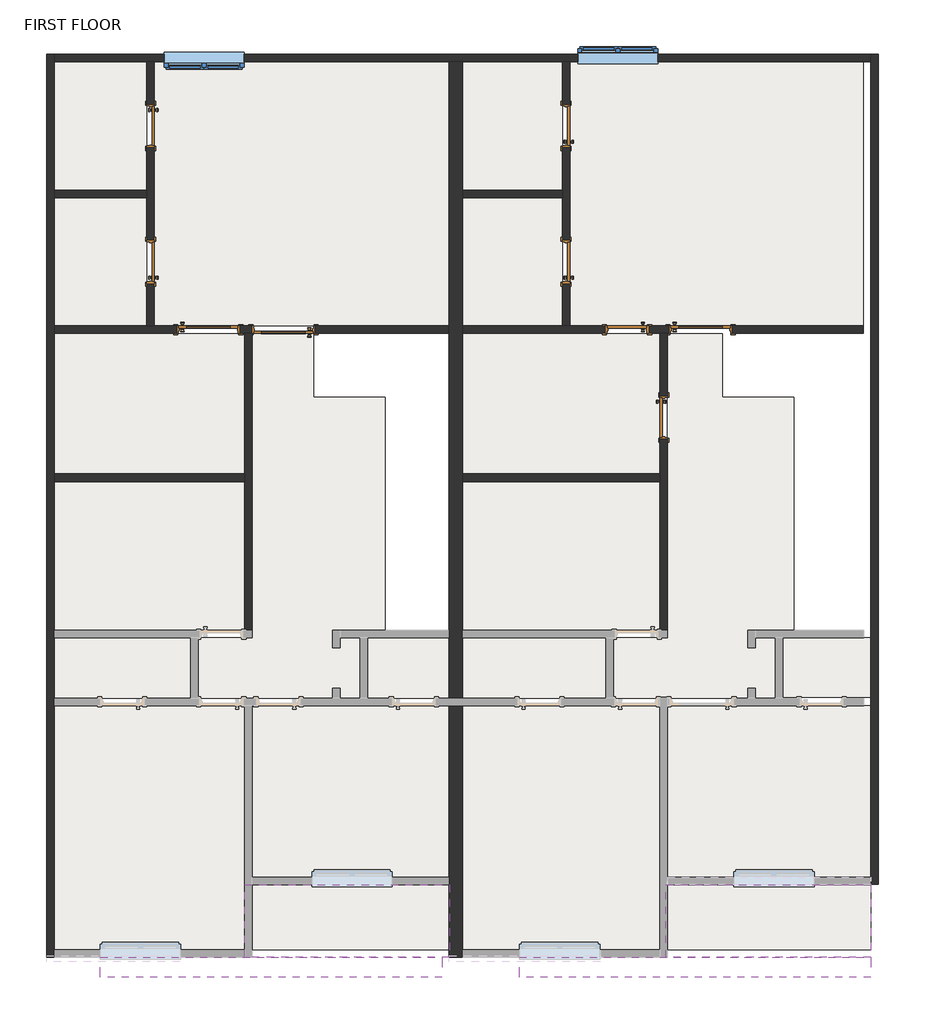
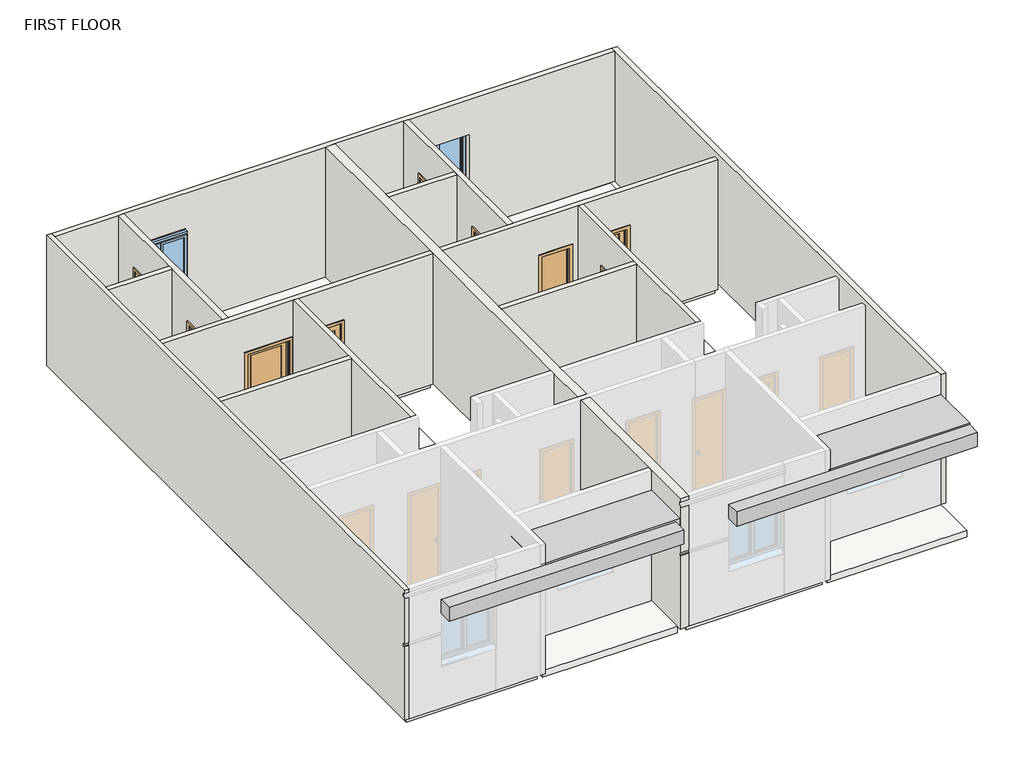
# One storey, part 2 of 2: 14 walls, 9 doors, 4 proxies, 2 slabs, 2 windows, 1 beam.
"""IFC4 building model written with IfcOpenShell, lengths in millimetres."""

from ifc_helpers import new_model, si_unit, frame, origin, place, context, project, spatial, polyline, outline, extrude, faceted_brep, transform, mapped, element, save
from components import w_shapes_w12x26_f1af6e5e, generic_models_1_generic_models_1_a2adb7c9, generic_models_2_generic_models_2_3446db89, generic_models_4_generic_models_1_d4ed459b, door_d4071c8b, door_c25f678d, door_03233f92, w2_0001_w2_3_7b164e2c

model = new_model("IFC4")

# Units and contexts
model_context = context("Model", 3, world=origin())
ifc_project = project(units=[si_unit("LENGTHUNIT", "METRE", prefix="MILLI")], contexts=[model_context])

# Site, building, storey
site = spatial("IfcSite", under=ifc_project)
building = spatial("IfcBuilding", under=site)
storey = spatial("IfcBuildingStorey", under=building, Name="FIRST FLOOR", Elevation=3352.8)

# Beam
placement = place(None, origin())
w_shapes_w12x26_shape = w_shapes_w12x26_f1af6e5e(model_context)
element("IfcBeam", 1, ObjectType="W Shapes : W12X26", at=placement, inside=storey, context=model_context, shape_type="MappedRepresentation", body=[
    mapped(w_shapes_w12x26_shape, transform((-13919.8007021, -597.2590801, 3197.86), x_axis=(0.0, 1.0, 0.0), y_axis=(-1.0, 0.0, 0.0), z_axis=(0.0, 0.0, 1.0))),
])

# Proxies
generic_models_1_generic_models_1_shape = generic_models_1_generic_models_1_a2adb7c9(model_context)
element("IfcBuildingElementProxy", 2, Name="Generic Models 1 : Generic Models 1", ObjectType="Generic Models 1 : Generic Models 1", at=placement, inside=storey, context=model_context, shape_type="MappedRepresentation", body=[
    mapped(generic_models_1_generic_models_1_shape, transform((0.0, 0.0, 0.0), x_axis=(1.0, 0.0, 0.0), y_axis=(0.0, 1.0, 0.0), z_axis=(0.0, 0.0, 1.0))),
])
generic_models_2_generic_models_2_shape = generic_models_2_generic_models_2_3446db89(model_context)
element("IfcBuildingElementProxy", 3, Name="Generic Models 2 : Generic Models 2", ObjectType="Generic Models 2 : Generic Models 2", at=placement, inside=storey, context=model_context, shape_type="MappedRepresentation", body=[
    mapped(generic_models_2_generic_models_2_shape, transform((0.0, 0.0, 0.0), x_axis=(1.0, 0.0, 0.0), y_axis=(0.0, 1.0, 0.0), z_axis=(0.0, 0.0, 1.0))),
])
element("IfcBuildingElementProxy", 4, Name="Generic Models 3 : Generic Models 2", ObjectType="Generic Models 3 : Generic Models 2", at=placement, inside=storey, context=model_context, shape_type="MappedRepresentation", body=[
    mapped(generic_models_2_generic_models_2_shape, transform((6400.8, 0.0, 0.0), x_axis=(1.0, 0.0, 0.0), y_axis=(0.0, 1.0, 0.0), z_axis=(0.0, 0.0, 1.0))),
])
generic_models_4_generic_models_1_shape = generic_models_4_generic_models_1_d4ed459b(model_context)
element("IfcBuildingElementProxy", 5, Name="Generic Models 4 : Generic Models 1", ObjectType="Generic Models 4 : Generic Models 1", at=placement, inside=storey, context=model_context, shape_type="MappedRepresentation", body=[
    mapped(generic_models_4_generic_models_1_shape, transform((6368.5786506, 0.0, 0.0), x_axis=(1.0, 0.0, 0.0), y_axis=(0.0, 1.0, 0.0), z_axis=(0.0, 0.0, 1.0))),
])

# Doors
door_shape = door_d4071c8b(model_context)
element("IfcDoor", 6, ObjectType="Door-Interior-Single-2_Panel-Wood : 36\" x 84\"", at=placement, inside=storey, context=model_context, shape_type="MappedRepresentation", body=[
    mapped(door_shape, transform((-14662.7507021, 4098.5659199, 3352.8), x_axis=(-1.0, 0.0, 0.0), y_axis=(0.0, -1.0, 0.0), z_axis=(0.0, 0.0, 1.0))),
])
element("IfcDoor", 7, ObjectType="Door-Interior-Single-2_Panel-Wood : 36\" x 84\"", at=placement, inside=storey, context=model_context, shape_type="MappedRepresentation", body=[
    mapped(door_shape, transform((-15805.7507021, 4104.9159199, 3352.8), x_axis=(1.0, 0.0, 0.0), y_axis=(0.0, 1.0, 0.0), z_axis=(0.0, 0.0, 1.0))),
])
element("IfcDoor", 8, ObjectType="Door-Interior-Single-2_Panel-Wood : 36\" x 84\"", at=placement, inside=storey, context=model_context, shape_type="MappedRepresentation", body=[
    mapped(door_shape, transform((-8325.4507021, 4104.9159199, 3352.8), x_axis=(1.0, 0.0, 0.0), y_axis=(0.0, 1.0, 0.0), z_axis=(0.0, 0.0, 1.0))),
])
door_2_shape = door_c25f678d(model_context)
element("IfcDoor", 9, ObjectType="Door-Interior-Single-Flush_Panel-Wood : 24\" x 84\"", at=placement, inside=storey, context=model_context, shape_type="MappedRepresentation", body=[
    mapped(door_2_shape, transform((-16678.8757021, 7197.3659199, 3352.8), x_axis=(0.0, -1.0, 0.0), y_axis=(1.0, 0.0, 0.0), z_axis=(0.0, 0.0, 1.0))),
])
door_3_shape = door_03233f92(model_context)
element("IfcDoor", 10, ObjectType="Door-Interior-Single-Flush_Panel-Wood : 24\" x 84\"", at=placement, inside=storey, context=model_context, shape_type="MappedRepresentation", body=[
    mapped(door_3_shape, transform((-16678.8757021, 5133.6159199, 3352.8), x_axis=(0.0, 1.0, 0.0), y_axis=(-1.0, 0.0, 0.0), z_axis=(0.0, 0.0, 1.0))),
])
element("IfcDoor", 11, ObjectType="Door-Interior-Single-Flush_Panel-Wood : 24\" x 84\"", at=placement, inside=storey, context=model_context, shape_type="MappedRepresentation", body=[
    mapped(door_3_shape, transform((-10366.9757021, 5133.6159199, 3352.8), x_axis=(0.0, 1.0, 0.0), y_axis=(-1.0, 0.0, 0.0), z_axis=(0.0, 0.0, 1.0))),
])
element("IfcDoor", 12, ObjectType="Door-Interior-Single-Flush_Panel-Wood : 24\" x 84\"", at=placement, inside=storey, context=model_context, shape_type="MappedRepresentation", body=[
    mapped(door_3_shape, transform((-10366.9757021, 7197.3659199, 3352.8), x_axis=(0.0, 1.0, 0.0), y_axis=(-1.0, 0.0, 0.0), z_axis=(0.0, 0.0, 1.0))),
])
element("IfcDoor", 13, ObjectType="Door-Interior-Single-Flush_Panel-Wood : 24\" x 84\"", at=placement, inside=storey, context=model_context, shape_type="MappedRepresentation", body=[
    mapped(door_3_shape, transform((-8887.4257021, 2768.2409199, 3352.8), x_axis=(0.0, -1.0, 0.0), y_axis=(1.0, 0.0, 0.0), z_axis=(0.0, 0.0, 1.0))),
])
element("IfcDoor", 14, ObjectType="Door-Interior-Single-Flush_Panel-Wood : 24\" x 84\"", at=placement, inside=storey, context=model_context, shape_type="MappedRepresentation", body=[
    mapped(door_3_shape, transform((-9443.0507021, 4104.9159199, 3352.8), x_axis=(-1.0, 0.0, 0.0), y_axis=(0.0, -1.0, 0.0), z_axis=(0.0, 0.0, 1.0))),
])

# Slabs
element("IfcSlab", 15, ObjectType="Generic - 12\" 2", at=placement, inside=storey, context=model_context, shape_type="SweptSolid", body=[
    extrude(outline(polyline([(-16739.2007021, 8172.0909199), (-16739.2007021, 6222.6409199), (-18148.9007021, 6222.6409199), (-18148.9007021, 8172.0909199), (-16739.2007021, 8172.0909199)])), frame((0.0, 0.0, 3200.4), z_axis=(0.0, 0.0, 1.0), x_axis=(1.0, 0.0, 0.0)), (0.0, 0.0, 1.0), 152.4),
    extrude(outline(polyline([(-16739.2007021, 6108.3409199), (-16739.2007021, 4158.8909199), (-18148.9007021, 4158.8909199), (-18148.9007021, 6108.3409199), (-16739.2007021, 6108.3409199)])), frame((0.0, 0.0, 3200.4), z_axis=(0.0, 0.0, 1.0), x_axis=(1.0, 0.0, 0.0)), (0.0, 0.0, 1.0), 152.4),
    extrude(outline(polyline([(-15253.3007021, 4044.5909199), (-15253.3007021, 1910.9909199), (-18148.9007021, 1910.9909199), (-18148.9007021, 4044.5909199), (-15253.3007021, 4044.5909199)])), frame((0.0, 0.0, 3200.4), z_axis=(0.0, 0.0, 1.0), x_axis=(1.0, 0.0, 0.0)), (0.0, 0.0, 1.0), 152.4),
    extrude(outline(polyline([(-15233.3480934, 1796.6909199), (-15233.3480934, -463.9090801), (-18148.9007021, -463.9090801), (-18148.9007021, 1796.6909199), (-15233.3480934, 1796.6909199)])), frame((0.0, 0.0, 3200.4), z_axis=(0.0, 0.0, 1.0), x_axis=(1.0, 0.0, 0.0)), (0.0, 0.0, 1.0), 152.4),
    extrude(outline(polyline([(-5849.8934009, 8172.0909199), (-5849.8934009, 4158.8909199), (-10313.0007021, 4158.8909199), (-10313.0007021, 8172.0909199), (-5849.8934009, 8172.0909199)])), frame((0.0, 0.0, 3200.4), z_axis=(0.0, 0.0, 1.0), x_axis=(1.0, 0.0, 0.0)), (0.0, 0.0, 1.0), 152.4),
    extrude(outline(polyline([(-10427.3007021, 6108.3409199), (-10427.3007021, 4158.8909199), (-11945.8934009, 4158.8909199), (-11945.8934009, 6108.3409199), (-10427.3007021, 6108.3409199)])), frame((0.0, 0.0, 3200.4), z_axis=(0.0, 0.0, 1.0), x_axis=(1.0, 0.0, 0.0)), (0.0, 0.0, 1.0), 152.4),
    extrude(outline(polyline([(-10427.3007021, 8172.0909199), (-10427.3007021, 6222.6409199), (-11945.8934009, 6222.6409199), (-11945.8934009, 8172.0909199), (-10427.3007021, 8172.0909199)])), frame((0.0, 0.0, 3200.4), z_axis=(0.0, 0.0, 1.0), x_axis=(1.0, 0.0, 0.0)), (0.0, 0.0, 1.0), 152.4),
    extrude(outline(polyline([(-12149.0934009, 8172.0909199), (-12149.0934009, 4158.8909199), (-16624.9007021, 4158.8909199), (-16624.9007021, 8172.0909199), (-12149.0934009, 8172.0909199)])), frame((0.0, 0.0, 3200.4), z_axis=(0.0, 0.0, 1.0), x_axis=(1.0, 0.0, 0.0)), (0.0, 0.0, 1.0), 152.4),
    extrude(outline(polyline([(-8941.4007021, 1796.6909199), (-8941.4007021, -463.9090801), (-11945.8934009, -463.9090801), (-11945.8934009, 1796.6909199), (-8941.4007021, 1796.6909199)])), frame((0.0, 0.0, 3200.4), z_axis=(0.0, 0.0, 1.0), x_axis=(1.0, 0.0, 0.0)), (0.0, 0.0, 1.0), 152.4),
    extrude(outline(polyline([(-8941.4007021, 1910.9909199), (-11945.8934009, 1910.9909199), (-11945.8934009, 4044.5909199), (-8941.4007021, 4044.5909199), (-8941.4007021, 1910.9909199)])), frame((0.0, 0.0, 3200.4), z_axis=(0.0, 0.0, 1.0), x_axis=(1.0, 0.0, 0.0)), (0.0, 0.0, 1.0), 152.4),
    extrude(outline(polyline([(-15253.300702, -5315.3090801), (-18148.9007021, -5315.3090801), (-18148.9007021, -1606.9090801), (-15253.300702, -1606.9090801), (-15253.300702, -5315.3090801)])), frame((0.0, 0.0, 3200.4), z_axis=(0.0, 0.0, 1.0), x_axis=(1.0, 0.0, 0.0)), (0.0, 0.0, 1.0), 152.4),
    extrude(outline(polyline([(-12149.0934009, -5315.3090801), (-15139.000702, -5315.3090801), (-15139.000702, -1606.9090801), (-12149.0934009, -1606.9090801), (-12149.0934009, -5315.3090801)])), frame((0.0, 0.0, 3200.4), z_axis=(0.0, 0.0, 1.0), x_axis=(1.0, 0.0, 0.0)), (0.0, 0.0, 1.0), 152.4),
])
element("IfcSlab", 16, ObjectType="Generic - 12\" 2", at=placement, inside=storey, context=model_context, shape_type="SweptSolid", body=[
    extrude(outline(polyline([(-8933.2454847, -5315.3090801), (-11945.8934009, -5315.3090801), (-11945.8934009, -1606.9090801), (-8933.2454847, -1606.9090801), (-8933.2454847, -5315.3090801)])), frame((0.0, 0.0, 3200.4), z_axis=(0.0, 0.0, 1.0), x_axis=(1.0, 0.0, 0.0)), (0.0, 0.0, 1.0), 152.4),
    extrude(outline(polyline([(-5742.8860997, -5315.3090801), (-8827.100702, -5315.3090801), (-8827.100702, -1606.9090801), (-5742.8860997, -1606.9090801), (-5742.8860997, -5315.3090801)])), frame((0.0, 0.0, 3200.4), z_axis=(0.0, 0.0, 1.0), x_axis=(1.0, 0.0, 0.0)), (0.0, 0.0, 1.0), 152.4),
    extrude(outline(polyline([(-5742.8860997, -578.2090801), (-5742.8860997, -1479.9090801), (-7074.5007021, -1479.9090801), (-7074.5007021, -578.2090801), (-5742.8860997, -578.2090801)])), frame((0.0, 0.0, 3200.4), z_axis=(0.0, 0.0, 1.0), x_axis=(1.0, 0.0, 0.0)), (0.0, 0.0, 1.0), 152.4),
    extrude(outline(polyline([(-9765.0954848, -578.2090801), (-9765.0954848, -1492.6090801), (-11945.8934009, -1492.6090801), (-11945.8934009, -578.2090801), (-9765.0954848, -578.2090801)])), frame((0.0, 0.0, 3200.4), z_axis=(0.0, 0.0, 1.0), x_axis=(1.0, 0.0, 0.0)), (0.0, 0.0, 1.0), 152.4),
    extrude(outline(polyline([(-16076.9954847, -578.2090801), (-16076.9954847, -1492.6090801), (-18148.9007021, -1492.6090801), (-18148.9007021, -578.2090801), (-16076.9954847, -578.2090801)])), frame((0.0, 0.0, 3200.4), z_axis=(0.0, 0.0, 1.0), x_axis=(1.0, 0.0, 0.0)), (0.0, 0.0, 1.0), 152.4),
    extrude(outline(polyline([(-12149.0934009, -578.2090801), (-12149.0934009, -1492.6090801), (-13386.4007021, -1492.6090801), (-13386.4007021, -578.2090801), (-12149.0934009, -578.2090801)])), frame((0.0, 0.0, 3200.4), z_axis=(0.0, 0.0, 1.0), x_axis=(1.0, 0.0, 0.0)), (0.0, 0.0, 1.0), 152.4),
    extrude(outline(polyline([(-15962.6954847, -578.2090801), (-15139.0007021, -578.2090801), (-15139.0007021, 4044.5909199), (-14205.5507021, 4044.5909199), (-14205.5507021, 3079.3909199), (-13119.7007021, 3079.3909199), (-13119.7007021, -463.9090801), (-13919.8007021, -463.9090801), (-13919.8007021, -730.6090801), (-13805.5007021, -730.6090801), (-13805.5007021, -578.2090801), (-13500.7007021, -578.2090801), (-13500.7007021, -1492.6090801), (-13805.5007021, -1492.6090801), (-13805.5007021, -1340.2090801), (-13919.8007021, -1340.2090801), (-13919.8007021, -1492.6090801), (-15962.6954847, -1492.6090801), (-15962.6954847, -578.2090801)])), frame((0.0, 0.0, 3200.4), z_axis=(0.0, 0.0, 1.0), x_axis=(1.0, 0.0, 0.0)), (0.0, 0.0, 1.0), 152.4),
    extrude(outline(polyline([(-9650.7954848, -578.2090801), (-8827.1007021, -578.2090801), (-8827.1007021, 4044.5909199), (-7996.544927, 4044.5909199), (-7996.544927, 3079.3909199), (-6911.2860997, 3079.3909199), (-6911.2860997, -463.9090801), (-7607.9007021, -463.9090801), (-7607.9007021, -730.6090801), (-7493.6007021, -730.6090801), (-7493.6007021, -578.2090801), (-7188.8007021, -578.2090801), (-7188.8007021, -1492.6090801), (-7493.6007021, -1492.6090801), (-7493.6007021, -1340.2090801), (-7607.9007021, -1340.2090801), (-7607.9007021, -1492.6090801), (-7830.1507021, -1492.6090801), (-9650.7954848, -1492.6090801), (-9650.7954848, -578.2090801)])), frame((0.0, 0.0, 3200.4), z_axis=(0.0, 0.0, 1.0), x_axis=(1.0, 0.0, 0.0)), (0.0, 0.0, 1.0), 152.4),
])

# Walls
element("IfcWall", 17, at=placement, inside=storey, context=model_context, shape_type="Brep", body=[
    faceted_brep([(-18263.2007021, 8286.3909199, 3352.8), (-18263.2007021, -5429.6090801, 3352.8), (-18263.2007021, -5429.6090801, 5072.38), (-18263.2007021, -5404.2090801, 5072.38), (-18263.2007021, -5404.2090801, 5140.1133333), (-18263.2007021, -5429.6090801, 5140.1133333), (-18263.2007021, -5429.6090801, 6248.4), (-18263.2007021, -5404.2090801, 6248.4), (-18263.2007021, -5404.2090801, 6316.1333333), (-18263.2007021, -5429.6090801, 6316.1333333), (-18263.2007021, -5429.6090801, 6400.8), (-18263.2007021, 8286.3909199, 6400.8), (-18148.9007021, -5429.6090801, 3352.8), (-18148.9007021, -5315.3090801, 3352.8), (-18148.9007021, -1606.9090801, 3352.8), (-18148.9007021, -1492.6090801, 3352.8), (-18148.9007021, -578.2090801, 3352.8), (-18148.9007021, -463.9090801, 3352.8), (-18148.9007021, 1796.6909199, 3352.8), (-18148.9007021, 1910.9909199, 3352.8), (-18148.9007021, 4044.5909199, 3352.8), (-18148.9007021, 4158.8909199, 3352.8), (-18148.9007021, 6108.3409199, 3352.8), (-18148.9007021, 6222.6409199, 3352.8), (-18148.9007021, 8172.0909199, 3352.8), (-18148.9007021, 8286.3909199, 3352.8), (-18148.9007021, 8286.3909199, 6400.8), (-18148.9007021, 8172.0909199, 6400.8), (-18148.9007021, 6222.6409199, 6400.8), (-18148.9007021, 6108.3409199, 6400.8), (-18148.9007021, 4158.8909199, 6400.8), (-18148.9007021, 4044.5909199, 6400.8), (-18148.9007021, 1910.9909199, 6400.8), (-18148.9007021, 1796.6909199, 6400.8), (-18148.9007021, -463.9090801, 6400.8), (-18148.9007021, -578.2090801, 6400.8), (-18148.9007021, -1492.6090801, 6400.8), (-18148.9007021, -1606.9090801, 6400.8), (-18148.9007021, -5315.3090801, 6400.8), (-18148.9007021, -5429.6090801, 6400.8), (-18148.9007021, -5429.6090801, 6316.1333333), (-18148.9007021, -5404.2090801, 6316.1333333), (-18148.9007021, -5404.2090801, 6248.4), (-18148.9007021, -5429.6090801, 6248.4), (-18148.9007021, -5429.6090801, 5140.1133333), (-18148.9007021, -5404.2090801, 5140.1133333), (-18148.9007021, -5404.2090801, 5072.38), (-18148.9007021, -5429.6090801, 5072.38)], [[[0, 1, 2, 3, 4, 5, 6, 7, 8, 9, 10, 11]], [[12, 13, 14, 15, 16, 17, 18, 19, 20, 21, 22, 23, 24, 25, 26, 27, 28, 29, 30, 31, 32, 33, 34, 35, 36, 37, 38, 39, 40, 41, 42, 43, 44, 45, 46, 47]], [[1, 0, 25, 24, 23, 22, 21, 20, 19, 18, 17, 16, 15, 14, 13, 12]], [[11, 10, 39, 38, 37, 36, 35, 34, 33, 32, 31, 30, 29, 28, 27, 26]], [[0, 11, 26, 25]], [[1, 12, 47, 2]], [[39, 10, 9, 40]], [[43, 6, 5, 44]], [[9, 8, 41, 40]], [[7, 6, 43, 42]], [[8, 7, 42, 41]], [[45, 4, 3, 46]], [[46, 3, 2, 47]], [[4, 45, 44, 5]]]),
])
element("IfcWall", 18, at=placement, inside=storey, context=model_context, shape_type="Brep", body=[
    faceted_brep([(-5628.5860997, -4318.3590801, 3352.8), (-5628.5860997, 8286.3909199, 3352.8), (-5628.5860997, 8286.3909199, 6400.8), (-5628.5860997, -4318.3590801, 6400.8), (-5742.8860997, -4318.3590801, 3352.8), (-5742.8860997, -4318.3590801, 6400.8), (-5742.8860997, -4215.4340831, 6400.8), (-5742.8860997, 8172.0909199, 6400.8), (-5742.8860997, 8286.3909199, 6400.8), (-5742.8860997, 8286.3909199, 3352.8), (-5742.8860997, 8172.0909199, 3352.8), (-5742.8860997, -4215.4340831, 3352.8)], [[[0, 1, 2, 3]], [[4, 5, 6, 7, 8, 9, 10, 11]], [[1, 0, 4, 11, 10, 9]], [[3, 2, 8, 7, 6, 5]], [[0, 3, 5, 4]], [[2, 1, 9, 8]]]),
])
element("IfcWall", 19, at=placement, inside=storey, context=model_context, shape_type="Brep", body=[
    faceted_brep([(-5742.8860997, 8286.3909199, 3352.8), (-18148.9007021, 8286.3909199, 3352.8), (-18148.9007021, 8286.3909199, 6400.8), (-5742.8860997, 8286.3909199, 6400.8), (-16478.8507021, 8286.3909199, 4352.8), (-15259.6507021, 8286.3909199, 4352.8), (-15259.6507021, 8286.3909199, 5572.0), (-16478.8507021, 8286.3909199, 5572.0), (-8973.1507021, 8286.3909199, 4352.8), (-8973.1507021, 8286.3909199, 5572.0), (-10192.3507021, 8286.3909199, 5572.0), (-10192.3507021, 8286.3909199, 4352.8), (-5742.8860997, 8172.0909199, 3352.8), (-5742.8860997, 8172.0909199, 6400.8), (-10313.0007021, 8172.0909199, 6400.8), (-10427.3007021, 8172.0909199, 6400.8), (-11945.8934009, 8172.0909199, 6400.8), (-12149.0934009, 8172.0909199, 6400.8), (-16624.9007021, 8172.0909199, 6400.8), (-16739.2007021, 8172.0909199, 6400.8), (-18148.9007021, 8172.0909199, 6400.8), (-18148.9007021, 8172.0909199, 3352.8), (-16739.2007021, 8172.0909199, 3352.8), (-16624.9007021, 8172.0909199, 3352.8), (-12149.0934009, 8172.0909199, 3352.8), (-11945.8934009, 8172.0909199, 3352.8), (-10427.3007021, 8172.0909199, 3352.8), (-10313.0007021, 8172.0909199, 3352.8), (-16478.8507021, 8172.0909199, 4352.8), (-16478.8507021, 8172.0909199, 5572.0), (-15259.6507021, 8172.0909199, 5572.0), (-15259.6507021, 8172.0909199, 4352.8), (-8973.1507021, 8172.0909199, 4352.8), (-10192.3507021, 8172.0909199, 4352.8), (-10192.3507021, 8172.0909199, 5572.0), (-8973.1507021, 8172.0909199, 5572.0)], [[[0, 1, 2, 3], [4, 5, 6, 7], [8, 9, 10, 11]], [[12, 13, 14, 15, 16, 17, 18, 19, 20, 21, 22, 23, 24, 25, 26, 27], [28, 29, 30, 31], [32, 33, 34, 35]], [[1, 0, 12, 27, 26, 25, 24, 23, 22, 21]], [[3, 2, 20, 19, 18, 17, 16, 15, 14, 13]], [[0, 3, 13, 12]], [[2, 1, 21, 20]], [[29, 28, 4, 7]], [[30, 29, 7, 6]], [[31, 30, 6, 5]], [[28, 31, 5, 4]], [[9, 8, 32, 35]], [[10, 9, 35, 34]], [[11, 10, 34, 33]], [[8, 11, 33, 32]]]),
])
element("IfcWall", 20, at=placement, inside=storey, context=model_context, shape_type="Brep", body=[
    faceted_brep([(-16739.2007021, 4158.8909199, 6400.8), (-16739.2007021, 6108.3409199, 6400.8), (-16739.2007021, 6222.6409199, 6400.8), (-16739.2007021, 8172.0909199, 6400.8), (-16739.2007021, 8172.0909199, 3352.8), (-16739.2007021, 7527.5659199, 3352.8), (-16739.2007021, 7527.5659199, 5511.8), (-16739.2007021, 6867.1659199, 5511.8), (-16739.2007021, 6867.1659199, 3352.8), (-16739.2007021, 6222.6409199, 3352.8), (-16739.2007021, 6108.3409199, 3352.8), (-16739.2007021, 5463.8159199, 3352.8), (-16739.2007021, 5463.8159199, 5511.8), (-16739.2007021, 4803.4159199, 5511.8), (-16739.2007021, 4803.4159199, 3352.8), (-16739.2007021, 4158.8909199, 3352.8), (-16624.9007021, 8172.0909199, 6400.8), (-16624.9007021, 4158.8909199, 6400.8), (-16624.9007021, 4158.8909199, 3352.8), (-16624.9007021, 4803.4159199, 3352.8), (-16624.9007021, 4803.4159199, 5511.8), (-16624.9007021, 5463.8159199, 5511.8), (-16624.9007021, 5463.8159199, 3352.8), (-16624.9007021, 6867.1659199, 3352.8), (-16624.9007021, 6867.1659199, 5511.8), (-16624.9007021, 7527.5659199, 5511.8), (-16624.9007021, 7527.5659199, 3352.8), (-16624.9007021, 8172.0909199, 3352.8)], [[[0, 1, 2, 3, 4, 5, 6, 7, 8, 9, 10, 11, 12, 13, 14, 15]], [[16, 17, 18, 19, 20, 21, 22, 23, 24, 25, 26, 27]], [[4, 27, 26, 5]], [[18, 15, 14, 19]], [[8, 23, 22, 11, 10, 9]], [[3, 2, 1, 0, 17, 16]], [[4, 3, 16, 27]], [[0, 15, 18, 17]], [[7, 24, 23, 8]], [[24, 7, 6, 25]], [[25, 6, 5, 26]], [[21, 12, 11, 22]], [[12, 21, 20, 13]], [[13, 20, 19, 14]]]),
])
element("IfcWall", 21, at=placement, inside=storey, context=model_context, shape_type="Brep", body=[
    faceted_brep([(-12149.0934009, 4044.5909199, 6400.8), (-15139.0007021, 4044.5909199, 6400.8), (-15253.3007021, 4044.5909199, 6400.8), (-18148.9007021, 4044.5909199, 6400.8), (-18148.9007021, 4044.5909199, 3352.8), (-16288.3507021, 4044.5909199, 3352.8), (-16288.3507021, 4044.5909199, 5511.8), (-15323.1507021, 4044.5909199, 5511.8), (-15323.1507021, 4044.5909199, 3352.8), (-15253.3007021, 4044.5909199, 3352.8), (-15145.3507021, 4044.5909199, 3352.8), (-15145.3507021, 4044.5909199, 5511.8), (-14180.1507021, 4044.5909199, 5511.8), (-14180.1507021, 4044.5909199, 3352.8), (-12149.0934009, 4044.5909199, 3352.8), (-18148.9007021, 4158.8909199, 6400.8), (-16739.2007021, 4158.8909199, 6400.8), (-16624.9007021, 4158.8909199, 6400.8), (-12149.0934009, 4158.8909199, 6400.8), (-12149.0934009, 4158.8909199, 3352.8), (-14180.1507021, 4158.8909199, 3352.8), (-14180.1507021, 4158.8909199, 5511.8), (-15145.3507021, 4158.8909199, 5511.8), (-15145.3507021, 4158.8909199, 3352.8), (-15323.1507021, 4158.8909199, 3352.8), (-15323.1507021, 4158.8909199, 5511.8), (-16288.3507021, 4158.8909199, 5511.8), (-16288.3507021, 4158.8909199, 3352.8), (-16624.9007021, 4158.8909199, 3352.8), (-16739.2007021, 4158.8909199, 3352.8), (-18148.9007021, 4158.8909199, 3352.8)], [[[0, 1, 2, 3, 4, 5, 6, 7, 8, 9, 10, 11, 12, 13, 14]], [[15, 16, 17, 18, 19, 20, 21, 22, 23, 24, 25, 26, 27, 28, 29, 30]], [[4, 30, 29, 28, 27, 5]], [[19, 14, 13, 20]], [[23, 10, 9, 8, 24]], [[3, 2, 1, 0, 18, 17, 16, 15]], [[4, 3, 15, 30]], [[0, 14, 19, 18]], [[22, 11, 10, 23]], [[11, 22, 21, 12]], [[12, 21, 20, 13]], [[7, 25, 24, 8]], [[25, 7, 6, 26]], [[26, 6, 5, 27]]]),
])
element("IfcWall", 22, at=placement, inside=storey, context=model_context, shape_type="SweptSolid", body=[
    extrude(outline(polyline([(-16739.2007021, 6108.3409199), (-18148.9007021, 6108.3409199), (-18148.9007021, 6222.6409199), (-16739.2007021, 6222.6409199), (-16739.2007021, 6108.3409199)])), frame((0.0, 0.0, 3352.8), z_axis=(0.0, 0.0, 1.0), x_axis=(1.0, 0.0, 0.0)), (0.0, 0.0, 1.0), 3048.0),
])
element("IfcWall", 23, at=placement, inside=storey, context=model_context, shape_type="SweptSolid", body=[
    extrude(outline(polyline([(-15253.3007021, 1796.6909199), (-18148.9007021, 1796.6909199), (-18148.9007021, 1910.9909199), (-15253.3007021, 1910.9909199), (-15253.3007021, 1796.6909199)])), frame((0.0, 0.0, 3352.8), z_axis=(0.0, 0.0, 1.0), x_axis=(1.0, 0.0, 0.0)), (0.0, 0.0, 1.0), 3048.0),
])
element("IfcWall", 24, at=placement, inside=storey, context=model_context, shape_type="Brep", body=[
    faceted_brep([(-15139.0007021, -463.9090801, 3352.8), (-15139.0007021, 4044.5909199, 3352.8), (-15139.0007021, 4044.5909199, 6400.8), (-15139.0007021, -463.9090801, 6400.8), (-15253.3007021, -463.9090801, 3352.8), (-15253.3007021, -463.9090801, 6400.8), (-15253.3007021, 1796.6909199, 6400.8), (-15253.3007021, 1910.9909199, 6400.8), (-15253.3007021, 4044.5909199, 6400.8), (-15253.3007021, 4044.5909199, 3352.8), (-15253.3007021, 1910.9909199, 3352.8), (-15253.3007021, 1796.6909199, 3352.8)], [[[0, 1, 2, 3]], [[4, 5, 6, 7, 8, 9, 10, 11]], [[1, 0, 4, 11, 10, 9]], [[3, 2, 8, 7, 6, 5]], [[0, 3, 5, 4]], [[2, 1, 9, 8]]]),
])
element("IfcWall", 25, at=placement, inside=storey, context=model_context, shape_type="Brep", body=[
    faceted_brep([(-12149.0934009, 8172.0909199, 6400.8), (-12149.0934009, 8172.0909199, 3352.8), (-12149.0934009, 4158.8909199, 3352.8), (-12149.0934009, 4044.5909199, 3352.8), (-12149.0934009, -463.9090801, 3352.8), (-12149.0934009, -578.2090801, 3352.8), (-12149.0934009, -1492.6090801, 3352.8), (-12149.0934009, -1492.6090801, 6400.8), (-12149.0934009, -578.2090801, 6400.8), (-12149.0934009, -463.9090801, 6400.8), (-12149.0934009, 4044.5909199, 6400.8), (-12149.0934009, 4158.8909199, 6400.8), (-11945.8934009, 8172.0909199, 3352.8), (-11945.8934009, 8172.0909199, 6400.8), (-11945.8934009, 6222.6409199, 6400.8), (-11945.8934009, 6108.3409199, 6400.8), (-11945.8934009, 4158.8909199, 6400.8), (-11945.8934009, 4044.5909199, 6400.8), (-11945.8934009, 1910.9909199, 6400.8), (-11945.8934009, 1796.6909199, 6400.8), (-11945.8934009, -463.9090801, 6400.8), (-11945.8934009, -578.2090801, 6400.8), (-11945.8934009, -1492.6090801, 6400.8), (-11945.8934009, -1492.6090801, 3352.8), (-11945.8934009, -578.2090801, 3352.8), (-11945.8934009, -463.9090801, 3352.8), (-11945.8934009, 1796.6909199, 3352.8), (-11945.8934009, 1910.9909199, 3352.8), (-11945.8934009, 4044.5909199, 3352.8), (-11945.8934009, 4158.8909199, 3352.8), (-11945.8934009, 6108.3409199, 3352.8), (-11945.8934009, 6222.6409199, 3352.8)], [[[0, 1, 2, 3, 4, 5, 6, 7, 8, 9, 10, 11]], [[12, 13, 14, 15, 16, 17, 18, 19, 20, 21, 22, 23, 24, 25, 26, 27, 28, 29, 30, 31]], [[1, 12, 31, 30, 29, 28, 27, 26, 25, 24, 23, 6, 5, 4, 3, 2]], [[13, 0, 11, 10, 9, 8, 7, 22, 21, 20, 19, 18, 17, 16, 15, 14]], [[1, 0, 13, 12]], [[7, 6, 23, 22]]]),
    faceted_brep([(-12149.0934009, -1606.9090801, 3352.8), (-12149.0934009, -4215.434083, 3352.8), (-12149.0934009, -4329.734083, 3352.8), (-12149.0934009, -5430.6582515, 3352.8), (-12149.0934009, -5430.6582515, 5072.38), (-12149.0934009, -5405.2582515, 5072.38), (-12149.0934009, -5405.2582515, 5140.1133333), (-12149.0934009, -5430.6582515, 5140.1133333), (-12149.0934009, -5430.6582515, 6248.4), (-12149.0934009, -5405.2582515, 6248.4), (-12149.0934009, -5405.2582515, 6316.1333333), (-12149.0934009, -5430.6582515, 6316.1333333), (-12149.0934009, -5430.6582515, 6400.8), (-12149.0934009, -4329.734083, 6400.8), (-12149.0934009, -4215.434083, 6400.8), (-12149.0934009, -1606.9090801, 6400.8), (-11945.8934009, -1606.9090801, 6400.8), (-11945.8934009, -5316.3582515, 6400.8), (-11945.8934009, -5430.6582515, 6400.8), (-11945.8934009, -5430.6582515, 6316.1333333), (-11945.8934009, -5405.2582515, 6316.1333333), (-11945.8934009, -5405.2582515, 6248.4), (-11945.8934009, -5430.6582515, 6248.4), (-11945.8934009, -5430.6582515, 5140.1133333), (-11945.8934009, -5405.2582515, 5140.1133333), (-11945.8934009, -5405.2582515, 5072.38), (-11945.8934009, -5430.6582515, 5072.38), (-11945.8934009, -5430.6582515, 3352.8), (-11945.8934009, -5316.3582515, 3352.8), (-11945.8934009, -1606.9090801, 3352.8)], [[[0, 1, 2, 3, 4, 5, 6, 7, 8, 9, 10, 11, 12, 13, 14, 15]], [[16, 17, 18, 19, 20, 21, 22, 23, 24, 25, 26, 27, 28, 29]], [[3, 2, 1, 0, 29, 28, 27]], [[15, 14, 13, 12, 18, 17, 16]], [[0, 15, 16, 29]], [[3, 27, 26, 4]], [[18, 12, 11, 19]], [[22, 8, 7, 23]], [[10, 20, 19, 11]], [[21, 9, 8, 22]], [[20, 10, 9, 21]], [[6, 24, 23, 7]], [[25, 5, 4, 26]], [[24, 6, 5, 25]]]),
])
element("IfcWall", 26, at=placement, inside=storey, context=model_context, shape_type="Brep", body=[
    faceted_brep([(-10427.3007021, 4158.8909199, 6400.8), (-10427.3007021, 6108.3409199, 6400.8), (-10427.3007021, 6222.6409199, 6400.8), (-10427.3007021, 8172.0909199, 6400.8), (-10427.3007021, 8172.0909199, 3352.8), (-10427.3007021, 7527.5659199, 3352.8), (-10427.3007021, 7527.5659199, 5511.8), (-10427.3007021, 6867.1659199, 5511.8), (-10427.3007021, 6867.1659199, 3352.8), (-10427.3007021, 6222.6409199, 3352.8), (-10427.3007021, 6108.3409199, 3352.8), (-10427.3007021, 5463.8159199, 3352.8), (-10427.3007021, 5463.8159199, 5511.8), (-10427.3007021, 4803.4159199, 5511.8), (-10427.3007021, 4803.4159199, 3352.8), (-10427.3007021, 4158.8909199, 3352.8), (-10313.0007021, 8172.0909199, 6400.8), (-10313.0007021, 4158.8909199, 6400.8), (-10313.0007021, 4158.8909199, 3352.8), (-10313.0007021, 4803.4159199, 3352.8), (-10313.0007021, 4803.4159199, 5511.8), (-10313.0007021, 5463.8159199, 5511.8), (-10313.0007021, 5463.8159199, 3352.8), (-10313.0007021, 6867.1659199, 3352.8), (-10313.0007021, 6867.1659199, 5511.8), (-10313.0007021, 7527.5659199, 5511.8), (-10313.0007021, 7527.5659199, 3352.8), (-10313.0007021, 8172.0909199, 3352.8)], [[[0, 1, 2, 3, 4, 5, 6, 7, 8, 9, 10, 11, 12, 13, 14, 15]], [[16, 17, 18, 19, 20, 21, 22, 23, 24, 25, 26, 27]], [[4, 27, 26, 5]], [[18, 15, 14, 19]], [[22, 11, 10, 9, 8, 23]], [[3, 2, 1, 0, 17, 16]], [[4, 3, 16, 27]], [[0, 15, 18, 17]], [[21, 12, 11, 22]], [[12, 21, 20, 13]], [[13, 20, 19, 14]], [[25, 6, 5, 26]], [[6, 25, 24, 7]], [[7, 24, 23, 8]]]),
])
element("IfcWall", 27, at=placement, inside=storey, context=model_context, shape_type="Brep", body=[
    faceted_brep([(-5849.8934009, 4044.5909199, 3352.8), (-5849.8934009, 4044.5909199, 6400.8), (-8827.1007021, 4044.5909199, 6400.8), (-8941.4007021, 4044.5909199, 6400.8), (-11945.8934009, 4044.5909199, 6400.8), (-11945.8934009, 4044.5909199, 3352.8), (-9773.2507021, 4044.5909199, 3352.8), (-9773.2507021, 4044.5909199, 5511.8), (-9112.8507021, 4044.5909199, 5511.8), (-9112.8507021, 4044.5909199, 3352.8), (-8941.4007021, 4044.5909199, 3352.8), (-8827.1007021, 4044.5909199, 3352.8), (-8808.0507021, 4044.5909199, 3352.8), (-8808.0507021, 4044.5909199, 5511.8), (-7842.8507021, 4044.5909199, 5511.8), (-7842.8507021, 4044.5909199, 3352.8), (-5849.8934009, 4158.8909199, 6400.8), (-5849.8934009, 4158.8909199, 3352.8), (-7842.8507021, 4158.8909199, 3352.8), (-7842.8507021, 4158.8909199, 5511.8), (-8808.0507021, 4158.8909199, 5511.8), (-8808.0507021, 4158.8909199, 3352.8), (-9112.8507021, 4158.8909199, 3352.8), (-9112.8507021, 4158.8909199, 5511.8), (-9773.2507021, 4158.8909199, 5511.8), (-9773.2507021, 4158.8909199, 3352.8), (-10313.0007021, 4158.8909199, 3352.8), (-10427.3007021, 4158.8909199, 3352.8), (-11945.8934009, 4158.8909199, 3352.8), (-11945.8934009, 4158.8909199, 6400.8), (-10427.3007021, 4158.8909199, 6400.8), (-10313.0007021, 4158.8909199, 6400.8)], [[[0, 1, 2, 3, 4, 5, 6, 7, 8, 9, 10, 11, 12, 13, 14, 15]], [[16, 17, 18, 19, 20, 21, 22, 23, 24, 25, 26, 27, 28, 29, 30, 31]], [[17, 0, 15, 18]], [[5, 28, 27, 26, 25, 6]], [[9, 22, 21, 12, 11, 10]], [[1, 0, 17, 16]], [[4, 3, 2, 1, 16, 31, 30, 29]], [[5, 4, 29, 28]], [[24, 7, 6, 25]], [[7, 24, 23, 8]], [[8, 23, 22, 9]], [[14, 19, 18, 15]], [[19, 14, 13, 20]], [[20, 13, 12, 21]]]),
])
element("IfcWall", 28, at=placement, inside=storey, context=model_context, shape_type="SweptSolid", body=[
    extrude(outline(polyline([(-10427.3007021, 6108.3409199), (-11945.8934009, 6108.3409199), (-11945.8934009, 6222.6409199), (-10427.3007021, 6222.6409199), (-10427.3007021, 6108.3409199)])), frame((0.0, 0.0, 3352.8), z_axis=(0.0, 0.0, 1.0), x_axis=(1.0, 0.0, 0.0)), (0.0, 0.0, 1.0), 3048.0),
])
element("IfcWall", 29, at=placement, inside=storey, context=model_context, shape_type="SweptSolid", body=[
    extrude(outline(polyline([(-8941.4007021, 1796.6909199), (-11945.8934009, 1796.6909199), (-11945.8934009, 1910.9909199), (-8941.4007021, 1910.9909199), (-8941.4007021, 1796.6909199)])), frame((0.0, 0.0, 3352.8), z_axis=(0.0, 0.0, 1.0), x_axis=(1.0, 0.0, 0.0)), (0.0, 0.0, 1.0), 3048.0),
])
element("IfcWall", 30, at=placement, inside=storey, context=model_context, shape_type="Brep", body=[
    faceted_brep([(-8827.1007021, 4044.5909199, 6400.8), (-8827.1007021, -463.9090801, 6400.8), (-8827.1007021, -463.9090801, 3352.8), (-8827.1007021, 2438.0409199, 3352.8), (-8827.1007021, 2438.0409199, 5511.8), (-8827.1007021, 3098.4409199, 5511.8), (-8827.1007021, 3098.4409199, 3352.8), (-8827.1007021, 4044.5909199, 3352.8), (-8941.4007021, -463.9090801, 6400.8), (-8941.4007021, 1796.6909199, 6400.8), (-8941.4007021, 1910.9909199, 6400.8), (-8941.4007021, 4044.5909199, 6400.8), (-8941.4007021, 4044.5909199, 3352.8), (-8941.4007021, 3098.4409199, 3352.8), (-8941.4007021, 3098.4409199, 5511.8), (-8941.4007021, 2438.0409199, 5511.8), (-8941.4007021, 2438.0409199, 3352.8), (-8941.4007021, 1910.9909199, 3352.8), (-8941.4007021, 1796.6909199, 3352.8), (-8941.4007021, -463.9090801, 3352.8)], [[[0, 1, 2, 3, 4, 5, 6, 7]], [[8, 9, 10, 11, 12, 13, 14, 15, 16, 17, 18, 19]], [[2, 19, 18, 17, 16, 3]], [[12, 7, 6, 13]], [[1, 0, 11, 10, 9, 8]], [[2, 1, 8, 19]], [[0, 7, 12, 11]], [[15, 4, 3, 16]], [[4, 15, 14, 5]], [[5, 14, 13, 6]]]),
])

# Windows
w2_0001_w2_3_shape = w2_0001_w2_3_7b164e2c(model_context)
element("IfcWindow", 31, ObjectType="w2.0001 : w2 3", at=placement, inside=storey, context=model_context, shape_type="MappedRepresentation", body=[
    mapped(w2_0001_w2_3_shape, transform((-15869.2507021, 8229.2409199, 3352.8), x_axis=(1.0, 0.0, 0.0), y_axis=(0.0, 1.0, 0.0), z_axis=(0.0, 0.0, 1.0))),
])
element("IfcWindow", 32, ObjectType="w2.0001 : w2 3", at=placement, inside=storey, context=model_context, shape_type="MappedRepresentation", body=[
    mapped(w2_0001_w2_3_shape, transform((-9582.7507021, 8229.2409199, 3352.8), x_axis=(-1.0, 0.0, 0.0), y_axis=(0.0, -1.0, 0.0), z_axis=(0.0, 0.0, 1.0))),
])

save(model, "model.ifc")

# Revit data of these elements
# Type "W Shapes : W12X26"
#   Section Name Key = "W12X26"
#   Assembly Code = "B10"
#   Width = 6.490"
#   Web Thickness = 0.230"
#   Web Fillet = 0.300"
#   Warping Constant = 607.00 in⁶
#   Torsional Moment of Inertia = 0.30 in⁴
#   Section Area = 7.65 in²
#   Plastic Modulus weak axis = 8.17 in³
#   Plastic Modulus strong axis = 37.20 in³
#   Perimeter = 4.116 ft²/ft
#   Nominal Weight = 26.00 lbf/ft
#   Moment of Inertia weak axis = 17.30 in⁴
#   Moment of Inertia strong axis = 204.00 in⁴
#   Height = 12.200"
#   Flange Thickness = 0.380"
#   Elastic Modulus weak axis = 5.34 in³
#   Elastic Modulus strong axis = 33.40 in³
#   Clear Web Height = 0' - 10 1/8"
#   Centroid Vertical = 6.100"
#   Centroid Horizontal = 3.245"
#   Bolt Spacing = 0' - 3 1/2"
#   Length [instance default] = 5' - 0"
#   Structural Material [instance default] = Steel ASTM A992
#   Principal Axes Angle = 0
# Type "Door-Interior-Single-2_Panel-Wood : 36\" x 84\""
#   Type Mark = "9"
#   Assembly Code = "C1020300"
#   Analytic Construction = "Wooden"
#   Top Rail = 0' - 4 11/16"
#   Thickness = 0' - 1 3/8"
#   Thermal Resistance (R) = 2.5876 (h·ft²·°F)/BTU
#   Swing Angle [instance default] = 90.00°
#   Stiles = 0' - 4 3/4"
#   Rough Width = 3' - 2"
#   Rough Height = 7' - 1"
#   Lock Rail = 0' - 7 1/2"
#   Height = 7' - 0"
#   Width = 3' - 0"
#   Heat Transfer Coefficient (U) = 0.3865 BTU/(h·ft²·°F)
#   Bottom Rail = 0' - 9 1/8"
#   Trim Material = Cherry
#   Panel Material = Cherry
#   Frame Material = Cherry
#   Door Handle Material = Aluminum
#   Visual Light Transmittance = 0
#   Solar Heat Gain Coefficient = 0
#   Wall Closure = (empty or 0)
#   Function = (empty or 0)
# Type "Door-Interior-Single-Flush_Panel-Wood : 24\" x 84\""
#   Type Mark = "10"
#   Assembly Code = "C1020300"
#   Analytic Construction = "Wooden"
#   Thickness = 0' - 1 3/8"
#   Thermal Resistance (R) = 2.5876 (h·ft²·°F)/BTU
#   Swing Angle [instance default] = 90.00°
#   Rough Width = 2' - 2"
#   Rough Height = 7' - 1"
#   Height = 7' - 0"
#   Width = 2' - 0"
#   Heat Transfer Coefficient (U) = 0.3865 BTU/(h·ft²·°F)
#   Trim Material = Cherry
#   Panel Material = Cherry
#   Frame Material = Cherry
#   Door Handle Material = Aluminum
#   Visual Light Transmittance = 0
#   Solar Heat Gain Coefficient = 0
#   Wall Closure = (empty or 0)
#   Function = (empty or 0)
# Type "Generic - 12\" 2"
#   Assembly Code = "B1010"
#   Function = 0
#   Layers, outside or top first: 0' - 6" "marble flooring" (function 1)
# Type
#   Assembly Code = "B2010"
# Type
#   Assembly Code = "B2010"
# Type "w2.0001 : w2 3"
#   Type Mark = "21"
#   Operation = "DoublePanelVertical"
#   Keynote = "16.05.01"
#   Analytic Construction = "<None>"
#   Rough Width = 4' - 0"
#   Rough Height = 4' - 0"
#   Rahmentiefe = 0' - 2.3622"
#   Rahmenhöhe unten = 0' - 3.14961"
#   Rahmehöhe oben = 0' - 3.14961"
#   Rahmenbreite = 0' - 2.3622"
#   Height = 4' - 0"
#   Flügeltiefe = 0' - 2.3622"
#   Flügelbreite = 0' - 2.3622"
#   Einbautiefe (von außen) [instance default] = 0' - 5.51181"
#   Width = 4' - 0"
#   Kippflügel [instance default] = yes
#   Drehflügel im Grundriß darstellen [instance default] = no
#   Drehflügel [instance default] = yes
#   Define Thermal Properties by = 1
#   Rahmen [instance default] = none
#   Glas [instance default] = none
#   Flügel [instance default] = none
#   Fensterbank aussen [instance default] = none
#   Fensterbank innen [instance default] = none
#   Wall Closure = (empty or 0)
# Element 1 (IfcBeam, "W Shapes : W12X26")
#   Structural Material = Steel ASTM A992
#   Phase Created = New Construction
#   Materials on its faces: "Steel ASTM A992"
# Element 2 (IfcBuildingElementProxy, "Generic Models 1 : Generic Models 1")
#   Phase Created = New Construction
# Element 3 (IfcBuildingElementProxy, "Generic Models 2 : Generic Models 2")
#   Phase Created = New Construction
# Element 4 (IfcBuildingElementProxy, "Generic Models 3 : Generic Models 2")
#   Phase Created = New Construction
# Element 5 (IfcBuildingElementProxy, "Generic Models 4 : Generic Models 1")
#   Phase Created = New Construction
# Elements 6, 7, 8 (IfcDoor, "Door-Interior-Single-2_Panel-Wood : 36\" x 84\"")
#   Swing Angle = 90.00°
#   Phase Created = New Construction
#   Materials on its faces: "Cherry", "Aluminum"
# Elements 9, 10, 11, 12, 13, 14 (IfcDoor, "Door-Interior-Single-Flush_Panel-Wood : 24\" x 84\"")
#   Swing Angle = 90.00°
#   Phase Created = New Construction
#   Materials on its faces: "Cherry", "Aluminum"
# Elements 15, 16 (IfcSlab, "Generic - 12\" 2")
#   Height Offset From Level = 0' - 0"
#   Phase Created = New Construction
#   Materials on its faces: "marble flooring"
# Element 17 (IfcWall)
#   Top Offset = 0' - 0"
#   Base Offset = 0' - 0"
#   wall height = 10' - 0"
#   Phase Created = New Construction
#   Base Constraint = FIRST FLOOR
#   Top Constraint = TOP OF ROOF
#   Materials on its faces: "red brown cladding", "Clad - White"
# Elements 18, 19 (IfcWall)
#   Top Offset = 0' - 0"
#   Base Offset = 0' - 0"
#   wall height = 10' - 0"
#   Phase Created = New Construction
#   Base Constraint = FIRST FLOOR
#   Top Constraint = TOP OF ROOF
#   Materials on its faces: "red brown cladding"
# Elements 20, 21, 22, 23, 24, 25, 26, 27, 28, 29, 30 (IfcWall)
#   Top Offset = 0' - 0"
#   Base Offset = 0' - 0"
#   wall height = 10' - 0"
#   Phase Created = New Construction
#   Base Constraint = FIRST FLOOR
#   Top Constraint = TOP OF ROOF
# Element 31 (IfcWindow, "w2.0001 : w2 3")
#   Mark = "6"
#   Einbautiefe (von außen) = 0' - 5.51181"
#   Kippflügel = yes
#   Drehflügel im Grundriß darstellen = no
#   Drehflügel = yes
#   Rahmen = none
#   Glas = none
#   Flügel = none
#   Fensterbank innen = none
#   Fensterbank aussen = none
#   Phase Created = New Construction
#   Materials on its faces: "Fenster - Kunststoff", "Fenster - Kunststoff weiss", "Glass", "Fenster - Holz"
# Element 32 (IfcWindow, "w2.0001 : w2 3")
#   Mark = "7"
#   Einbautiefe (von außen) = 0' - 5.51181"
#   Kippflügel = yes
#   Drehflügel im Grundriß darstellen = no
#   Drehflügel = yes
#   Rahmen = none
#   Glas = none
#   Flügel = none
#   Fensterbank innen = none
#   Fensterbank aussen = none
#   Phase Created = New Construction
#   Materials on its faces: "Fenster - Kunststoff", "Fenster - Kunststoff weiss", "Glass", "Fenster - Holz"
# Materials
#   "Steel ASTM A992": class "Metal", colour RGB 199 199 199, transparency 0, Description = "Structural steel 50ksi", Cost = 0
#   "Cherry": class "Wood", colour RGB 226 177 128, transparency 0, Description = "Prunus Serotina", Cost = 0
#   "Aluminum": class "Metal", colour RGB 247 247 247, transparency 0, Description = "Aluminum 6061", Cost = 0
#   "marble flooring": class "Generic", colour RGB 120 120 120, transparency 0, Cost = 0
#   "red brown cladding": class "Generic", colour RGB 151 67 57, transparency 0, Cost = 0
#   "Clad - White": class "Wood", colour RGB 242 242 238, transparency 0, Cost = 0
#   "Fenster - Kunststoff": colour RGB 249 249 249, transparency 0
#   "Fenster - Kunststoff weiss": colour RGB 249 249 249, transparency 0
#   "Glass": class "Glass", colour RGB 0 128 192, transparency 0.75, Description = "Soda Lime Glass", Cost = 0
#   "Fenster - Holz": colour RGB 216 135 75, transparency 0
